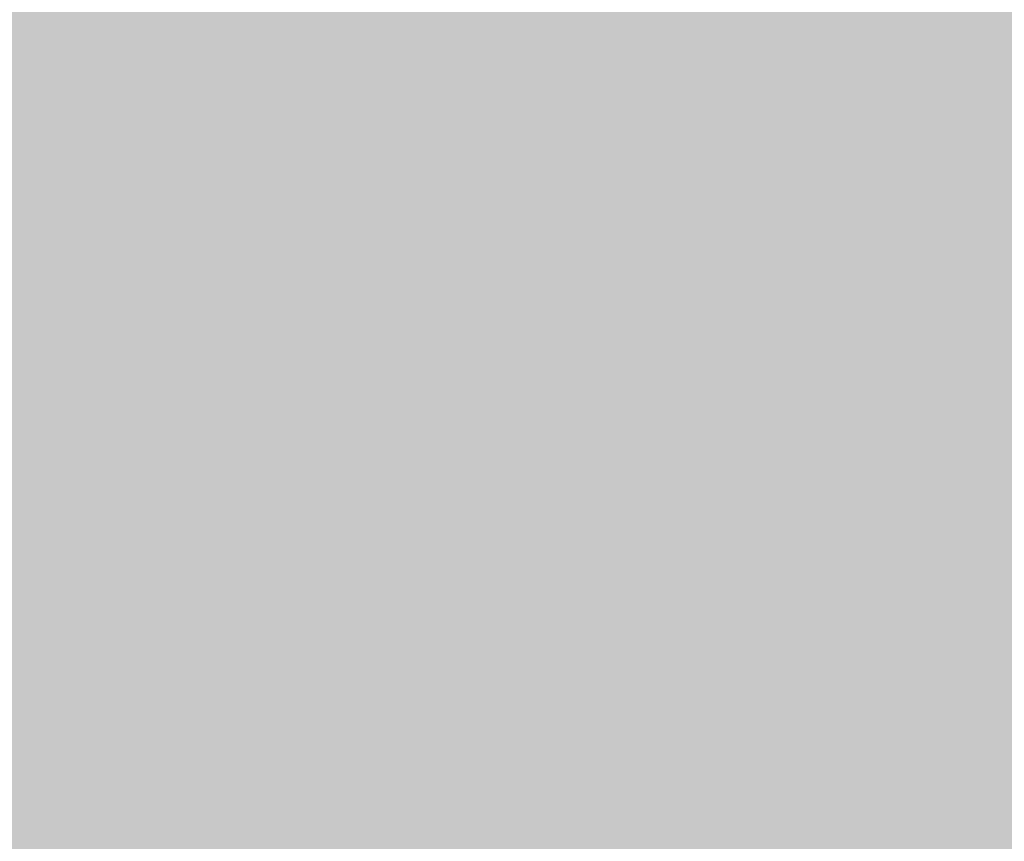
# Model space of a CAD drawing. Units: feet. Extents: x 3168 to 4724, y 827 to 1477.
# Tile 137 of 256: x 3301.12983 to 3301.14682, y 1099.00068 to 1099.01485. Entities that reach past the tile are written whole.
import ezdxf

# ---------------------------------------------------------------- set-up
doc = ezdxf.new("R2010")
doc.units = ezdxf.units.FT
doc.layers.add('A-ELEV', color=7, linetype='Continuous', lineweight=35)
doc.layers.add('A-ELEV-PATT', color=8, linetype='Continuous', lineweight=13)

msp = doc.modelspace()

# ---------------------------------------------------------------- hatches: boundary and pattern name
at = {"layer": 'A-ELEV-PATT'}
h = msp.add_hatch(color=256, dxfattribs=at)
h.dxf.hatch_style = 1
edge = h.paths.add_edge_path()
edge.add_ellipse((3552.905762, 979.220141), major_axis=(36.744924, 0), ratio=0.484848485, start_angle=0, end_angle=360)
edge = h.paths.add_edge_path()
edge.add_ellipse((3559.891637, 929.252282), major_axis=(36.744924, 0), ratio=0.484848485, start_angle=0, end_angle=360)
edge = h.paths.add_edge_path()
edge.add_line((3299.31681, 1198.606081), (3479.916714, 1198.606081))
edge.add_line((3479.916714, 1198.606081), (3479.916714, 1209.86857))
edge.add_spline(control_points=[(3479.916714, 1209.86857), (3464.301157, 1209.86857), (3448.685601, 1209.86857), (3410.949139, 1209.86857), (3388.828234, 1209.86857), (3355.646876, 1209.86857), (3344.586423, 1209.86857), (3327.995745, 1209.86857), (3322.465518, 1209.86857), (3314.170179, 1209.86857), (3311.405066, 1209.86857), (3307.257396, 1209.86857), (3305.874839, 1209.86857), (3303.801005, 1209.86857), (3303.109726, 1209.86857), (3302.072809, 1209.86857), (3301.72717, 1209.86857), (3301.208711, 1209.86857), (3301.035891, 1209.86857), (3300.776662, 1209.86857), (3300.690252, 1209.86857), (3300.560638, 1209.86857), (3300.517433, 1209.86857), (3300.452625, 1209.86857), (3300.431023, 1209.86857), (3300.398619, 1209.86857), (3300.387818, 1209.86857), (3300.366216, 1209.86857), (3300.345676, 1209.86857), (3300.345548, 1209.86857), (3300.345505, 1209.86857), (3300.343304, 1209.86857), (3300.341146, 1209.868571), (3300.337909, 1209.868571), (3300.33683, 1209.868572), (3300.333942, 1209.868573), (3300.332133, 1209.868574), (3300.325515, 1209.868577), (3300.320706, 1209.868581), (3300.310925, 1209.868592), (3300.305952, 1209.868598), (3300.290511, 1209.868623), (3300.280045, 1209.868646), (3300.232425, 1209.868777), (3300.195298, 1209.868954), (3299.951068, 1209.870608), (3299.744824, 1209.874326), (3299.436827, 1209.883257), (3299.334389, 1209.886792), (3299.181079, 1209.89292), (3299.130033, 1209.895099), (3298.652217, 1209.916801), (3298.22946, 1209.945718), (3297.601631, 1210.002367), (3297.393404, 1210.023464), (3297.082652, 1210.058309), (3296.979332, 1210.070458), (3296.292954, 1210.154861), (3295.718148, 1210.243356), (3294.868717, 1210.39885), (3294.5877, 1210.454478), (3294.169341, 1210.543349), (3294.030415, 1210.573878), (3291.707149, 1211.1012), (3289.65359, 1211.813435), (3285.776259, 1213.563988), (3283.95141, 1214.603478), (3280.512159, 1216.98008), (3278.897241, 1218.317592), (3276.379914, 1220.829489), (3275.416042, 1221.917738), (3274.039342, 1223.7077), (3273.581043, 1224.349535), (3273.143228, 1225.016316)], knot_values=[39.119033, 39.119033, 39.119033, 39.119033, 39.286353, 39.286353, 39.523379, 39.523379, 39.641892, 39.641892, 39.701148, 39.701148, 39.730777, 39.730777, 39.745591, 39.745591, 39.752998, 39.752998, 39.756701, 39.756701, 39.758553, 39.758553, 39.759479, 39.759479, 39.759942, 39.759942, 39.760173, 39.760173, 39.760289, 39.760289, 39.760405, 39.760405, 39.760463, 39.760463, 39.763389, 39.763389, 39.764851, 39.764851, 39.767304, 39.767304, 39.773825, 39.773825, 39.78057, 39.78057, 39.79477, 39.79477, 39.845194, 39.845194, 40.126715, 40.126715, 40.267476, 40.267476, 40.337856, 40.337856, 40.927023, 40.927023, 41.221606, 41.221606, 41.368898, 41.368898, 42.202622, 42.202622, 42.619485, 42.619485, 42.827916, 42.827916, 46.118323, 46.118323, 49.408731, 49.408731, 52.699139, 52.699139, 54.927489, 54.927489, 56.104228, 56.104228, 56.104228, 56.104228], weights=[1, 1, 1, 1, 1, 1, 1, 1, 1, 1, 1, 1, 1, 1, 1, 1, 1, 1, 1, 1, 1, 1, 1, 1, 1, 1, 1, 1, 1, 1, 1, 1, 1, 1, 1, 1, 1, 1, 1, 1, 1, 1, 1, 1, 1, 1, 1, 1, 1, 1, 1, 1, 1, 1, 1, 1, 1, 1, 1, 1, 1, 1, 1, 1, 1, 1, 1, 1, 1, 1, 1, 1, 1, 1], degree=3, periodic=0)
edge.add_line((3273.143228, 1225.016316), (3273.143228, 1099.016316))
edge.add_line((3273.143228, 1099.016316), (3299.31681, 1099.016316))
edge.add_line((3299.31681, 1099.016316), (3299.31681, 1198.606081))
edge = h.paths.add_edge_path()
edge.add_line((3304.758443, 1324.15806), (3479.916714, 1324.15806))
edge.add_line((3479.916714, 1324.15806), (3479.916714, 1335.714618))
edge.add_line((3479.916714, 1335.714618), (3269.161628, 1335.714618))
edge.add_spline(control_points=[(3269.161628, 1335.714618), (3264.024231, 1335.714618), (3258.364118, 1328.958189), (3259.264311, 1323.900274)], knot_values=[0, 0, 0, 0, 15.412191, 15.412191, 15.412191, 15.412191], degree=3, periodic=0)
edge.add_line((3259.264311, 1323.900274), (3265.516849, 1288.769135))
edge.add_line((3265.516849, 1288.769135), (3275.265103, 1261.545626))
edge.add_line((3275.265103, 1261.545626), (3304.758443, 1261.545626))
edge.add_line((3304.758443, 1261.545626), (3304.758443, 1324.15806))
h = msp.add_hatch(color=256, dxfattribs=at)
h.dxf.hatch_style = 1
h.paths.add_polyline_path([(3384.525247, 1099.016316), (3335.029168, 1099.016316), (3299.31681, 1099.016316), (3273.143228, 1099.016316), (3217.565364, 1099.016316), (3168.069285, 827.11626), (3335.029168, 827.11626)])

# ---------------------------------------------------------------- linework, layer by layer
at = {"layer": 'A-ELEV'}
msp.add_open_spline([(3808.5202, 1099.016316), (3808.5202, 1141.413235), (3808.5202, 1183.810154), (3808.5202, 1226.635324), (3808.5202, 1227.063576), (3808.5202, 1227.491828), (3811.491871, 1248.994673), (3814.463542, 1270.497518), (3817.46523, 1292.217564), (3817.495247, 1292.434764), (3817.525264, 1292.651964), (3817.572801, 1310.106748), (3817.620339, 1327.561532), (3817.667877, 1345.016316), (3817.667877, 1345.457962), (3817.667877, 1345.899608), (3817.667877, 1346.456047), (3817.667877, 1346.57084), (3817.667877, 1346.752887), (3817.667877, 1346.820142), (3817.667877, 1346.93487), (3817.667877, 1346.982345), (3817.667877, 1347.038587), (3817.667877, 1347.047356), (3817.667877, 1347.073661), (3817.667877, 1347.059303), (3817.667877, 1347.061545), (3817.667876, 1347.062667), (3817.667875, 1347.066031), (3817.667874, 1347.068274), (3817.66787, 1347.075001), (3817.667866, 1347.079486), (3817.667849, 1347.092937), (3817.667833, 1347.101902), (3817.667766, 1347.12879), (3817.667699, 1347.146705), (3817.667432, 1347.200421), (3817.667165, 1347.236192), (3817.6661, 1347.343385), (3817.665038, 1347.414686), (3817.660812, 1347.628095), (3817.656608, 1347.769708), (3817.63997, 1348.192487), (3817.623509, 1348.471586), (3817.559094, 1349.300067), (3817.496121, 1349.840588), (3817.255432, 1351.424156), (3817.026318, 1352.428785), (3816.306871, 1354.888914), (3815.743745, 1356.268727), (3814.463959, 1358.81921), (3813.746413, 1359.990968), (3812.195838, 1362.172343), (3811.362245, 1363.182124), (3809.588836, 1365.069009), (3808.648816, 1365.946105), (3806.654262, 1367.579616), (3805.599702, 1368.336154), (3803.352891, 1369.722327), (3802.160535, 1370.352386), (3799.600813, 1371.453586), (3798.232688, 1371.925481), (3795.280084, 1372.634624), (3793.693148, 1372.872068), (3791.869441, 1372.92648), (3791.740861, 1372.92922), (3791.353371, 1372.934101), (3791.092707, 1372.932901), (3790.304116, 1372.915068), (3789.769543, 1372.884195), (3789.20919, 1372.830236), (3789.190622, 1372.828424), (3789.134892, 1372.822912), (3789.097705, 1372.819137), (3789.048445, 1372.814008), (3789.0364, 1372.812743), (3789.000256, 1372.808918), (3788.976147, 1372.806325), (3788.949405, 1372.803404), (3788.946786, 1372.803118), (3788.942567, 1372.802655), (3788.940967, 1372.80248), (3788.938572, 1372.802217), (3788.937777, 1372.802129), (3788.935391, 1372.801867), (3788.867535, 1372.794402), (3788.756866, 1372.782228), (3788.701532, 1372.776141), (3788.53553, 1372.75788), (3788.424861, 1372.745707), (3788.092856, 1372.709185), (3787.871519, 1372.684837), (3787.207509, 1372.611793), (3786.764835, 1372.563097), (3785.436814, 1372.417009), (3784.551467, 1372.319617), (3781.895425, 1372.027442), (3780.12473, 1371.832658), (3774.812646, 1371.248307), (3771.271256, 1370.858739), (3760.647088, 1369.690037), (3753.56431, 1368.910902), (3732.315973, 1366.573498), (3718.150416, 1365.015228), (3694.006758, 1362.359326), (3684.028657, 1361.261694), (3674.050557, 1360.164062), (3664.600662, 1360.164062), (3655.150767, 1360.164062), (3626.801081, 1360.164062), (3607.901291, 1360.164062), (3551.20192, 1360.164062), (3513.40234, 1360.164062), (3467.725182, 1360.164062), (3459.847604, 1360.164062), (3436.214873, 1360.164062), (3420.459718, 1360.164062), (3373.194255, 1360.164062), (3341.683946, 1360.164062), (3302.848162, 1360.164062), (3295.522686, 1360.164062), (3286.038292, 1360.164062), (3283.879372, 1360.164062), (3277.402613, 1360.164062), (3273.084773, 1360.164062), (3267.732851, 1360.164062), (3266.698768, 1360.164062), (3263.59652, 1360.164062), (3261.528355, 1360.164062), (3259.236943, 1360.164062), (3259.013697, 1360.164062), (3258.343958, 1360.164062), (3257.897466, 1360.164062), (3257.430998, 1360.164062), (3257.411022, 1360.164062), (3257.370573, 1360.164062), (3257.37547, 1360.164062), (3257.374598, 1360.164062), (3257.373937, 1360.164062), (3257.371956, 1360.164062), (3257.370635, 1360.164061), (3257.366673, 1360.16406), (3257.364032, 1360.164059), (3257.356109, 1360.164053), (3257.350828, 1360.164047), (3257.334987, 1360.164023), (3257.32443, 1360.163998), (3257.292769, 1360.163899), (3257.271676, 1360.163799), (3257.208439, 1360.163398), (3257.166337, 1360.162995), (3257.040206, 1360.161388), (3256.956349, 1360.159783), (3256.705504, 1360.153393), (3256.53924, 1360.147036), (3256.04357, 1360.121916), (3255.717296, 1360.097102), (3254.752446, 1360.000481), (3254.127968, 1359.906513), (3252.180067, 1359.525332), (3250.941574, 1359.143991), (3248.670175, 1358.24329), (3247.635739, 1357.723834), (3245.732632, 1356.603471), (3244.863388, 1356.00206), (3243.253108, 1354.742865), (3242.511972, 1354.084731), (3240.751052, 1352.344781), (3239.800961, 1351.229574), (3238.087769, 1348.87244), (3237.324685, 1347.630355), (3235.98251, 1344.971632), (3235.402205, 1343.554907), (3234.591081, 1340.815458), (3234.310882, 1339.54355), (3233.97649, 1336.802561), (3233.922113, 1335.330877), (3234.148916, 1332.591269), (3234.349529, 1331.367201), (3234.719893, 1329.999367), (3234.752423, 1329.883362), (3234.853619, 1329.534797), (3234.925892, 1329.301685), (3235.024836, 1329.002552), (3235.046924, 1328.936928), (3235.077639, 1328.847239), (3235.085924, 1328.823198), (3235.110939, 1328.751064), (3235.127828, 1328.702962), (3235.147992, 1328.646242), (3235.151059, 1328.637632), (3235.156096, 1328.623526), (3235.158061, 1328.61803), (3235.160209, 1328.61203), (3235.165612, 1328.596943), (3235.180099, 1328.556486), (3235.190263, 1328.528101), (3235.220756, 1328.442946), (3235.241084, 1328.386176), (3235.302069, 1328.215865), (3235.342726, 1328.102325), (3235.464696, 1327.761704), (3235.54601, 1327.534623), (3235.78995, 1326.853381), (3235.952577, 1326.39922), (3236.440459, 1325.036736), (3236.765713, 1324.128414), (3237.741475, 1321.403446), (3238.391983, 1319.586801), (3240.343508, 1314.136866), (3241.644525, 1310.503576), (3245.547574, 1299.603706), (3248.149607, 1292.337126), (3255.955706, 1270.537385), (3261.159772, 1256.004225), (3267.387618, 1238.612001), (3268.411397, 1235.752937), (3269.510378, 1232.683864), (3269.585579, 1232.473854), (3269.706612, 1232.135851), (3269.752444, 1232.007857), (3269.827329, 1231.79873), (3269.856382, 1231.717595), (3269.906325, 1231.578122), (3269.927215, 1231.519782), (3269.972468, 1231.393406), (3269.996831, 1231.325368), (3270.026503, 1231.242506), (3270.031811, 1231.227681), (3270.040282, 1231.204024), (3270.039224, 1231.206979), (3270.039359, 1231.206601), (3270.039427, 1231.206412), (3270.03963, 1231.205846), (3270.039765, 1231.205468), (3270.040171, 1231.204335), (3270.040442, 1231.203579), (3270.041254, 1231.201313), (3270.041796, 1231.199802), (3270.04342, 1231.195269), (3270.044504, 1231.192248), (3270.047756, 1231.183185), (3270.049926, 1231.177145), (3270.056442, 1231.159028), (3270.060793, 1231.146957), (3270.073867, 1231.110761), (3270.082613, 1231.086656), (3270.108936, 1231.014413), (3270.1266, 1230.96635), (3270.179934, 1230.822457), (3270.215947, 1230.726923), (3270.325323, 1230.441508), (3270.400026, 1230.252811), (3270.629249, 1229.691444), (3270.788883, 1229.323501), (3271.286488, 1228.238319), (3271.6431, 1227.539755), (3272.775859, 1225.515277), (3273.614169, 1224.260502), (3275.416042, 1221.917738), (3276.379914, 1220.829489), (3278.897241, 1218.317592), (3280.512159, 1216.98008), (3283.95141, 1214.603478), (3285.776259, 1213.563988), (3289.65359, 1211.813435), (3291.707149, 1211.1012), (3294.030415, 1210.573878), (3294.169341, 1210.543349), (3294.5877, 1210.454478), (3294.868717, 1210.39885), (3295.718148, 1210.243356), (3296.292954, 1210.154861), (3296.979332, 1210.070458), (3297.082652, 1210.058309), (3297.393404, 1210.023464), (3297.601631, 1210.002367), (3298.22946, 1209.945718), (3298.652217, 1209.916801), (3299.130033, 1209.895099), (3299.181079, 1209.89292), (3299.334389, 1209.886792), (3299.436827, 1209.883257), (3299.744824, 1209.874326), (3299.951068, 1209.870608), (3300.195298, 1209.868954), (3300.232425, 1209.868777), (3300.280045, 1209.868646), (3300.290511, 1209.868623), (3300.305952, 1209.868598), (3300.310925, 1209.868592), (3300.320706, 1209.868581), (3300.325515, 1209.868577), (3300.332133, 1209.868574), (3300.333942, 1209.868573), (3300.33683, 1209.868572), (3300.337909, 1209.868571), (3300.341146, 1209.868571), (3300.343304, 1209.86857), (3300.345505, 1209.86857), (3300.345548, 1209.86857), (3300.345676, 1209.86857), (3300.366216, 1209.86857), (3300.387818, 1209.86857), (3300.398619, 1209.86857), (3300.431023, 1209.86857), (3300.452625, 1209.86857), (3300.517433, 1209.86857), (3300.560638, 1209.86857), (3300.690252, 1209.86857), (3300.776662, 1209.86857), (3301.035891, 1209.86857), (3301.208711, 1209.86857), (3301.72717, 1209.86857), (3302.072809, 1209.86857), (3303.109726, 1209.86857), (3303.801005, 1209.86857), (3305.874839, 1209.86857), (3307.257396, 1209.86857), (3311.405066, 1209.86857), (3314.170179, 1209.86857), (3322.465518, 1209.86857), (3327.995745, 1209.86857), (3344.586423, 1209.86857), (3355.646876, 1209.86857), (3388.828234, 1209.86857), (3410.949139, 1209.86857), (3477.311855, 1209.86857), (3521.553665, 1209.86857), (3566.836184, 1209.86857), (3567.876892, 1209.86857), (3570.999017, 1209.86857), (3573.080433, 1209.86857), (3575.781396, 1209.86857), (3576.400943, 1209.86857), (3577.295821, 1209.86857), (3577.571152, 1209.86857), (3578.397146, 1209.86857), (3578.947808, 1209.86857), (3579.756491, 1209.86857), (3580.014511, 1209.86857), (3580.342737, 1209.86857), (3580.326865, 1209.86857), (3580.32717, 1209.86857), (3580.327323, 1209.86857), (3580.327781, 1209.86857), (3580.328086, 1209.86857), (3580.329002, 1209.86857), (3580.329613, 1209.86857), (3580.331445, 1209.86857), (3580.332667, 1209.86857), (3580.336332, 1209.868569), (3580.338775, 1209.868567), (3580.346107, 1209.868563), (3580.350995, 1209.868558), (3580.365663, 1209.86854), (3580.375445, 1209.868522), (3580.404801, 1209.868449), (3580.424386, 1209.868376), (3580.483183, 1209.868085), (3580.522437, 1209.867793), (3580.640361, 1209.866624), (3580.719195, 1209.865454), (3580.956315, 1209.860766), (3581.115222, 1209.85607), (3581.594164, 1209.83723), (3581.916419, 1209.818331), (3582.889947, 1209.742428), (3583.547986, 1209.666169), (3585.531827, 1209.360617), (3586.867216, 1209.053886), (3589.471545, 1208.252472), (3590.740241, 1207.757852), (3591.995451, 1207.158802), (3592.057809, 1207.12874), (3592.244242, 1207.037954), (3592.367676, 1206.976632), (3592.73528, 1206.790359), (3592.976752, 1206.663101), (3593.244539, 1206.516441), (3593.274731, 1206.499825), (3593.365115, 1206.449839), (3593.425113, 1206.416333), (3593.604314, 1206.315285), (3593.722725, 1206.247211), (3593.857212, 1206.168398), (3593.874362, 1206.158319), (3593.925741, 1206.128041), (3593.959899, 1206.107798), (3594.062086, 1206.046899), (3594.129827, 1206.006074), (3594.208436, 1205.958171), (3594.219683, 1205.951304), (3594.253391, 1205.930686), (3594.275819, 1205.916917), (3594.342972, 1205.875536), (3594.387563, 1205.847853), (3594.433616, 1205.81905), (3594.435256, 1205.818024), (3594.440175, 1205.814946), (3594.443453, 1205.812894), (3594.447123, 1205.810594), (3594.447516, 1205.810348), (3594.448695, 1205.80961), (3594.449481, 1205.809117), (3594.450366, 1205.808562), (3594.450466, 1205.8085), (3594.4506, 1205.808415), (3594.467399, 1205.797887), (3594.493269, 1205.781674), (3594.506204, 1205.773568), (3594.545008, 1205.749248), (3594.570878, 1205.733035), (3594.648487, 1205.684396), (3594.700226, 1205.651969), (3594.855444, 1205.554691), (3594.958922, 1205.489839), (3595.269357, 1205.295282), (3595.476314, 1205.165577), (3596.097185, 1204.776463), (3596.511099, 1204.517054), (3597.752841, 1203.738826), (3598.580669, 1203.220007), (3601.064152, 1201.663551), (3602.719807, 1200.625914), (3607.686774, 1197.513002), (3610.998085, 1195.437727), (3620.932018, 1189.211903), (3627.55464, 1185.061354), (3647.422507, 1172.609707), (3660.667751, 1164.308608), (3700.403484, 1139.405313), (3726.893973, 1122.803116), (3757.205715, 1103.806052), (3761.02697, 1101.411184), (3764.848224, 1099.016316), (3745.328271, 1099.016316), (3725.808319, 1099.016316), (3706.288366, 1099.016316), (3706.288366, 1108.453237), (3706.288366, 1117.890158), (3706.288366, 1127.327079), (3710.750754, 1127.327079), (3715.213143, 1127.327079), (3719.675531, 1127.327079)], degree=3, knots=[0, 0, 0, 0, 0.982037, 0.982037, 0.991957, 0.991957, 0.991957, 1.966522, 1.966522, 1.976367, 1.976367, 1.976367, 2.976367, 2.976367, 2.976367, 3.00169, 3.00169, 3.008272, 3.008272, 3.012129, 3.012129, 3.014851, 3.014851, 3.015353, 3.015353, 3.016359, 3.016359, 3.017365, 3.017365, 3.019376, 3.019376, 3.023398, 3.023398, 3.031442, 3.031442, 3.047531, 3.047531, 3.079708, 3.079708, 3.144063, 3.144063, 3.272772, 3.272772, 3.53019, 3.53019, 4.045026, 4.045026, 5.074698, 5.074698, 6.700878, 6.700878, 8.327058, 8.327058, 9.953238, 9.953238, 11.579418, 11.579418, 13.205598, 13.205598, 14.831778, 14.831778, 16.457958, 16.457958, 18.084138, 18.084138, 18.206872, 18.206872, 18.45234, 18.45234, 18.943275, 18.943275, 18.960093, 18.960093, 18.993729, 18.993729, 19.00461, 19.00461, 19.026374, 19.026374, 19.028737, 19.028737, 19.03018, 19.03018, 19.030897, 19.030897, 19.032332, 19.032332, 19.033766, 19.033766, 19.036636, 19.036636, 19.042374, 19.042374, 19.053851, 19.053851, 19.076805, 19.076805, 19.122714, 19.122714, 19.21453, 19.21453, 19.398163, 19.398163, 19.765429, 19.765429, 20.024128, 20.024128, 20.024128, 20.092031, 20.092031, 20.227836, 20.227836, 20.499446, 20.499446, 20.556051, 20.556051, 20.66926, 20.66926, 20.895678, 20.895678, 20.948316, 20.948316, 20.963829, 20.963829, 20.994855, 20.994855, 21.002285, 21.002285, 21.017146, 21.017146, 21.01875, 21.01875, 21.021959, 21.021959, 21.022102, 21.022102, 21.022249, 21.022249, 21.022708, 21.022708, 21.023627, 21.023627, 21.025464, 21.025464, 21.029138, 21.029138, 21.036486, 21.036486, 21.051183, 21.051183, 21.080575, 21.080575, 21.139361, 21.139361, 21.256932, 21.256932, 21.492073, 21.492073, 21.962356, 21.962356, 23.01002, 23.01002, 24.057684, 24.057684, 25.105348, 25.105348, 26.153011, 26.153011, 27.776787, 27.776787, 29.400562, 29.400562, 31.024337, 31.024337, 32.278801, 32.278801, 33.533265, 33.533265, 34.467568, 34.467568, 34.553971, 34.553971, 34.726776, 34.726776, 34.775309, 34.775309, 34.793079, 34.793079, 34.82862, 34.82862, 34.834979, 34.834979, 34.839039, 34.839039, 34.839411, 34.839411, 34.840285, 34.840285, 34.842034, 34.842034, 34.845531, 34.845531, 34.852525, 34.852525, 34.866512, 34.866512, 34.894488, 34.894488, 34.950439, 34.950439, 35.062342, 35.062342, 35.286147, 35.286147, 35.733758, 35.733758, 35.821815, 35.821815, 35.828283, 35.828283, 35.832225, 35.832225, 35.834724, 35.834724, 35.836521, 35.836521, 35.838617, 35.838617, 35.839073, 35.839073, 35.839345, 35.839345, 35.839617, 35.839617, 35.840161, 35.840161, 35.841249, 35.841249, 35.843425, 35.843425, 35.847778, 35.847778, 35.856482, 35.856482, 35.873891, 35.873891, 35.908709, 35.908709, 35.978345, 35.978345, 36.117617, 36.117617, 36.396161, 36.396161, 36.953248, 36.953248, 38.067423, 38.067423, 40.295772, 40.295772, 42.524122, 42.524122, 45.81453, 45.81453, 49.104937, 49.104937, 52.395345, 52.395345, 52.603776, 52.603776, 53.020639, 53.020639, 53.854363, 53.854363, 54.001655, 54.001655, 54.296238, 54.296238, 54.885405, 54.885405, 54.955785, 54.955785, 55.096546, 55.096546, 55.378067, 55.378067, 55.42849, 55.42849, 55.442691, 55.442691, 55.449436, 55.449436, 55.455957, 55.455957, 55.458409, 55.458409, 55.459872, 55.459872, 55.462798, 55.462798, 55.462856, 55.462856, 55.462972, 55.462972, 55.463088, 55.463088, 55.463319, 55.463319, 55.463782, 55.463782, 55.464708, 55.464708, 55.46656, 55.46656, 55.470263, 55.470263, 55.47767, 55.47767, 55.492484, 55.492484, 55.522112, 55.522112, 55.581369, 55.581369, 55.699882, 55.699882, 55.936907, 55.936907, 56.410959, 56.410959, 56.42211, 56.42211, 56.444413, 56.444413, 56.451051, 56.451051, 56.454001, 56.454001, 56.459901, 56.459901, 56.462666, 56.462666, 56.463418, 56.463418, 56.464171, 56.464171, 56.465675, 56.465675, 56.468684, 56.468684, 56.474702, 56.474702, 56.486738, 56.486738, 56.51081, 56.51081, 56.558955, 56.558955, 56.655243, 56.655243, 56.847821, 56.847821, 57.232975, 57.232975, 58.003284, 58.003284, 59.543901, 59.543901, 62.625137, 62.625137, 68.787607, 68.787607, 74.950078, 74.950078, 75.27336, 75.27336, 75.919923, 75.919923, 77.213051, 77.213051, 77.377769, 77.377769, 77.707206, 77.707206, 78.366079, 78.366079, 78.462532, 78.462532, 78.655436, 78.655436, 79.041245, 79.041245, 79.105735, 79.105735, 79.234714, 79.234714, 79.492672, 79.492672, 79.502197, 79.502197, 79.521249, 79.521249, 79.523534, 79.523534, 79.528103, 79.528103, 79.528682, 79.528682, 79.528885, 79.528885, 79.529089, 79.529089, 79.529495, 79.529495, 79.530308, 79.530308, 79.531935, 79.531935, 79.535187, 79.535187, 79.541693, 79.541693, 79.554704, 79.554704, 79.580725, 79.580725, 79.632769, 79.632769, 79.736856, 79.736856, 79.94503, 79.94503, 80.361377, 80.361377, 80.421435, 80.421435, 80.421435, 81.421435, 81.421435, 81.421435, 82.421435, 82.421435, 82.421435, 83.421435, 83.421435, 83.421435, 83.421435], dxfattribs=at)

doc.saveas('drawing.dxf')
